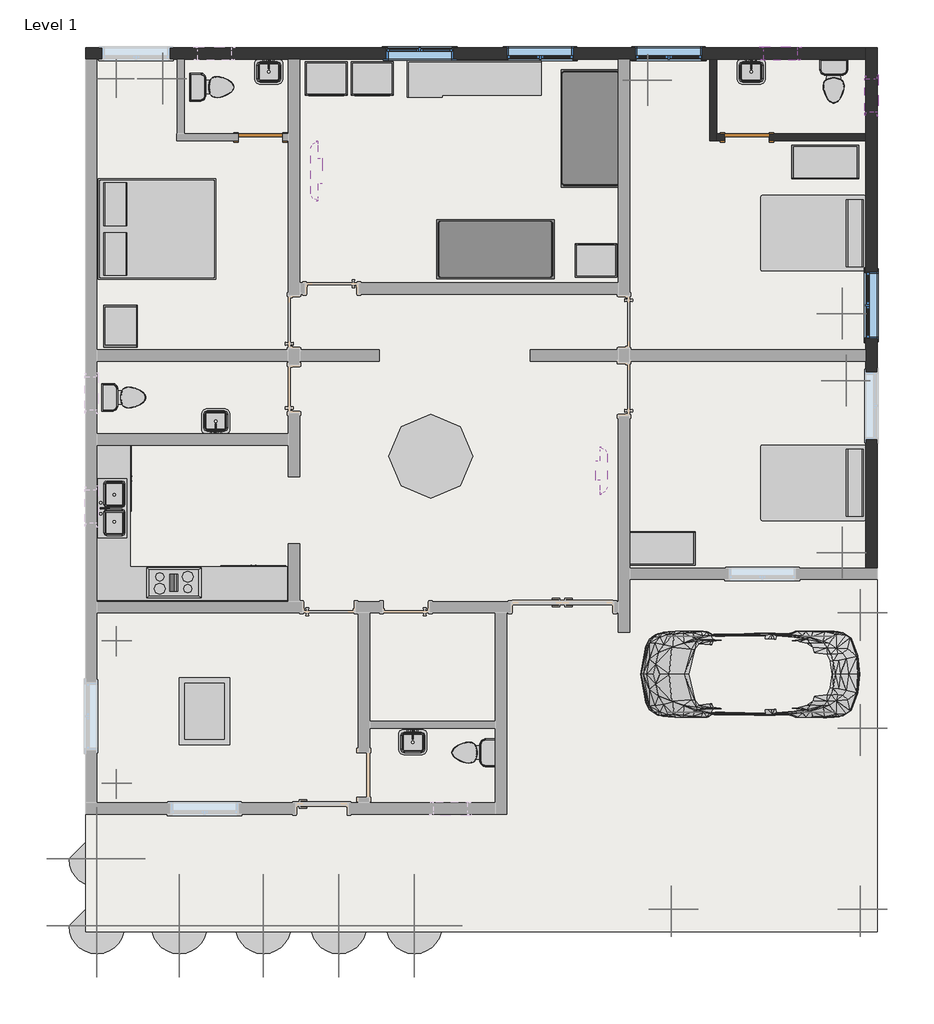
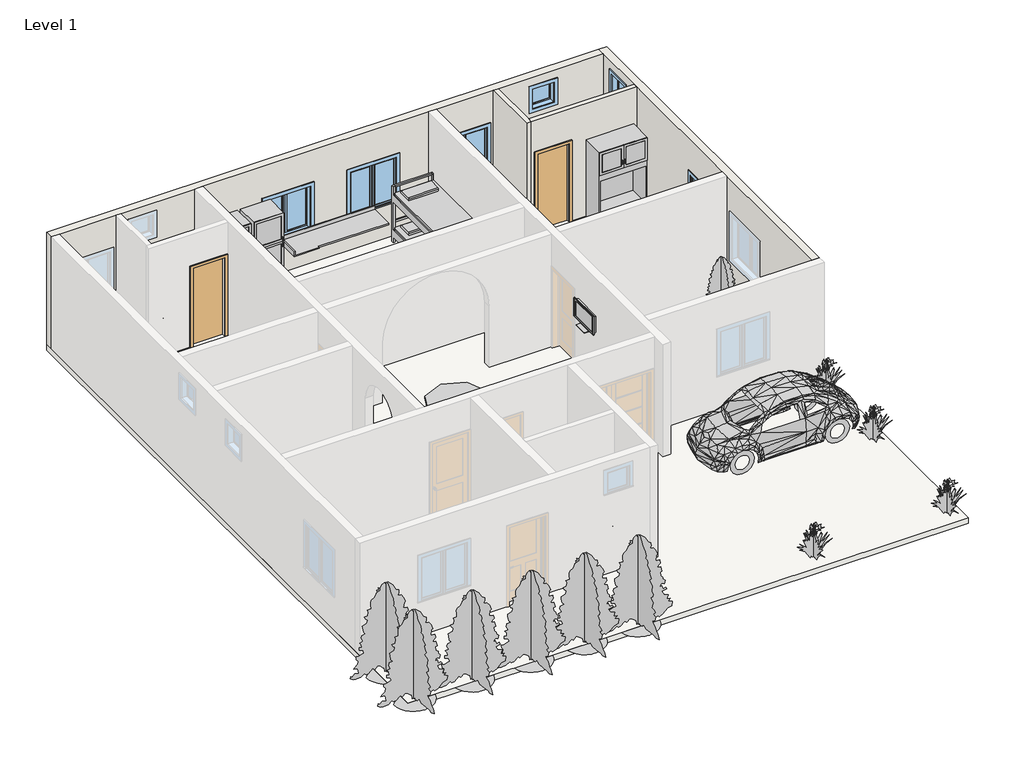
# One storey, part 2 of 2: 20 furniture elements, 18 geographic elements, 9 flow terminals, 6 windows, 4 walls, 2 doors, 2 proxies, 1 slab.
"""IFC4 building model written with IfcOpenShell, lengths in millimetres."""

from ifc_helpers import new_model, si_unit, frame, origin, place, context, project, spatial, polyline, outline, extrude, faceted_brep, transform, mapped, element, save
from components import cook_top_4_unit_30_51a8ed57, rpc_beetle_rpc_beetle_3ce7ba48, door_01e03998, door_af63d1be, flow_terminal_a53be723, flow_terminal_62a433f7, toilet_domestic_3d_toilet_domestic_3d_f7549cf7, toilet_domestic_3d_toilet_domestic_3d_183bbd19, furniture_7e5e5cd5, furniture_5816963c, furniture_2b620373, furniture_0253826f, furniture_3ce93e2e, furniture_bc267eac, furniture_56245f3a, furniture_7a3aaa4f, furniture_4da399da, furniture_bbcc68ce, tall_cabinet_2_door_built_in_3_fb6977ac, furniture_4aee2c20, furniture_7f1a6afb, rpc_plant_tropical_55f6ff97, rpc_tree_conifer_9dfc94cb, rpc_tree_conifer_8_e62f4ae5, rpc_tree_conifer_chinese_juniper_7_393522d0, rpc_tree_conifer_eastern_hemlock_25_66632feb, window_0862ab64, window_e41d21a6

model = new_model("IFC4")

# Units and contexts
model_context = context("Model", 3, world=origin())
ifc_project = project(units=[si_unit("LENGTHUNIT", "METRE", prefix="MILLI")], contexts=[model_context])

# Site, building, storey
site = spatial("IfcSite", under=ifc_project)
building = spatial("IfcBuilding", under=site)
storey = spatial("IfcBuildingStorey", under=building, Name="Level 1", Elevation=0.0)

# Proxies
placement = place(None, origin())
cook_top_4_unit_30_shape = cook_top_4_unit_30_51a8ed57(model_context)
element("IfcBuildingElementProxy", 1, Name="Cook Top-4 Unit : 30'", ObjectType="Cook Top-4 Unit : 30'", at=placement, inside=storey, context=model_context, shape_type="MappedRepresentation", body=[
    mapped(cook_top_4_unit_30_shape, transform((-1417.9231918, 1904.1987331, 152.4), x_axis=(1.0, 0.0, 0.0), y_axis=(0.0, 1.0, 0.0), z_axis=(0.0, 0.0, 1.0))),
])
rpc_beetle_rpc_beetle_shape = rpc_beetle_rpc_beetle_3ce7ba48(model_context)
element("IfcBuildingElementProxy", 2, Name="RPC Beetle : RPC Beetle", ObjectType="RPC Beetle : RPC Beetle", at=placement, inside=storey, context=model_context, shape_type="MappedRepresentation", body=[
    mapped(rpc_beetle_rpc_beetle_shape, transform((10291.4768082, 240.4987331, 0.0), x_axis=(0.0, 1.0, 0.0), y_axis=(-1.0, 0.0, 0.0), z_axis=(0.0, 0.0, 1.0))),
])

# Doors
door_shape = door_01e03998(model_context)
element("IfcDoor", 3, ObjectType="Door-Single-Panel : 32\" x 84\"", at=placement, inside=storey, context=model_context, shape_type="MappedRepresentation", body=[
    mapped(door_shape, transform((156.8768082, 9994.0987331, 0.0), x_axis=(1.0, 0.0, 0.0), y_axis=(0.0, 1.0, 0.0), z_axis=(0.0, 0.0, 1.0))),
])
door_2_shape = door_af63d1be(model_context)
element("IfcDoor", 4, ObjectType="Door-Single-Panel : 32\" x 84\"", at=placement, inside=storey, context=model_context, shape_type="MappedRepresentation", body=[
    mapped(door_2_shape, transform((8996.0768082, 9994.0987331, 0.0), x_axis=(-1.0, 0.0, 0.0), y_axis=(0.0, -1.0, 0.0), z_axis=(0.0, 0.0, 1.0))),
])

# Flow terminals
flow_terminal_shape = flow_terminal_a53be723(model_context)
element("IfcFlowTerminal", 5, ObjectType="Sink Kitchen-Double : 42\" x 21\"", at=placement, inside=storey, context=model_context, shape_type="MappedRepresentation", body=[
    mapped(flow_terminal_shape, transform((-2533.1777907, 3240.0622298, 0.0), x_axis=(0.0, 1.0, 0.0), y_axis=(-1.0, 0.0, 0.0), z_axis=(0.0, 0.0, 1.0))),
])
flow_terminal_2_shape = flow_terminal_62a433f7(model_context)
element("IfcFlowTerminal", 6, ObjectType="Sink Vanity-Square : 20\" x 18\"", at=placement, inside=storey, context=model_context, shape_type="MappedRepresentation", body=[
    mapped(flow_terminal_2_shape, transform((-640.2339512, 4789.4441342, 0.0), x_axis=(-1.0000000000000002, 0.0, 0.0), y_axis=(0.0, -1.0000000000000002, 0.0), z_axis=(0.0, 0.0, 1.0))),
])
element("IfcFlowTerminal", 7, ObjectType="Sink Vanity-Square : 20\" x 18\"", at=placement, inside=storey, context=model_context, shape_type="MappedRepresentation", body=[
    mapped(flow_terminal_2_shape, transform((293.5875676, 11236.353332, 0.0), x_axis=(1.0, 0.0, 0.0), y_axis=(0.0, 1.0, 0.0), z_axis=(0.0, 0.0, 1.0))),
])
element("IfcFlowTerminal", 8, ObjectType="Sink Vanity-Square : 20\" x 18\"", at=placement, inside=storey, context=model_context, shape_type="MappedRepresentation", body=[
    mapped(flow_terminal_2_shape, transform((9056.5875676, 11236.353332, 0.0), x_axis=(1.0, 0.0, 0.0), y_axis=(0.0, 1.0, 0.0), z_axis=(0.0, 0.0, 1.0))),
])
element("IfcFlowTerminal", 9, ObjectType="Sink Vanity-Square : 20\" x 18\"", at=placement, inside=storey, context=model_context, shape_type="MappedRepresentation", body=[
    mapped(flow_terminal_2_shape, transform((2909.7875676, -942.946668, 0.0), x_axis=(1.0, 0.0, 0.0), y_axis=(0.0, 1.0, 0.0), z_axis=(0.0, 0.0, 1.0))),
])
toilet_domestic_3d_toilet_domestic_3d_shape = toilet_domestic_3d_toilet_domestic_3d_f7549cf7(model_context)
toilet_domestic_3d_toilet_domestic_3d_2_shape = toilet_domestic_3d_toilet_domestic_3d_183bbd19(model_context)
element("IfcFlowTerminal", 10, ObjectType="Toilet-Domestic-3D : Toilet-Domestic-3D", at=placement, inside=storey, context=model_context, shape_type="MappedRepresentation", body=[
    mapped(toilet_domestic_3d_toilet_domestic_3d_shape, transform((3941.4768082, -1181.9012669, 0.0), x_axis=(0.0, -1.0, 0.0), y_axis=(1.0, 0.0, 0.0), z_axis=(0.0, 0.0, 1.0))),
    mapped(toilet_domestic_3d_toilet_domestic_3d_2_shape, transform((3941.4768082, -1181.9012669, 0.0), x_axis=(0.0, -1.0, 0.0), y_axis=(1.0, 0.0, 0.0), z_axis=(0.0, 0.0, 1.0))),
])
element("IfcFlowTerminal", 11, ObjectType="Toilet-Domestic-3D : Toilet-Domestic-3D", at=placement, inside=storey, context=model_context, shape_type="MappedRepresentation", body=[
    mapped(toilet_domestic_3d_toilet_domestic_3d_shape, transform((-630.5231918, 10908.4987331, 0.0), x_axis=(0.0, 1.0000000000000004, 0.0), y_axis=(-1.0000000000000004, 0.0, 0.0), z_axis=(0.0, 0.0, 1.0))),
    mapped(toilet_domestic_3d_toilet_domestic_3d_2_shape, transform((-630.5231918, 10908.4987331, 0.0), x_axis=(0.0, 1.0000000000000004, 0.0), y_axis=(-1.0000000000000004, 0.0, 0.0), z_axis=(0.0, 0.0, 1.0))),
])
element("IfcFlowTerminal", 12, ObjectType="Toilet-Domestic-3D : Toilet-Domestic-3D", at=placement, inside=storey, context=model_context, shape_type="MappedRepresentation", body=[
    mapped(toilet_domestic_3d_toilet_domestic_3d_shape, transform((10570.8768082, 10921.8027057, 0.0), x_axis=(1.0000000000000004, 0.0, 0.0), y_axis=(0.0, 1.0000000000000004, 0.0), z_axis=(0.0, 0.0, 1.0))),
    mapped(toilet_domestic_3d_toilet_domestic_3d_2_shape, transform((10570.8768082, 10921.8027057, 0.0), x_axis=(1.0000000000000004, 0.0, 0.0), y_axis=(0.0, 1.0000000000000004, 0.0), z_axis=(0.0, 0.0, 1.0))),
])
element("IfcFlowTerminal", 13, ObjectType="Toilet-Domestic-3D : Toilet-Domestic-3D", at=placement, inside=storey, context=model_context, shape_type="MappedRepresentation", body=[
    mapped(toilet_domestic_3d_toilet_domestic_3d_shape, transform((-2230.7231918, 5269.6987331, 0.0), x_axis=(0.0, 1.0, 0.0), y_axis=(-1.0, 0.0, 0.0), z_axis=(0.0, 0.0, 1.0))),
    mapped(toilet_domestic_3d_toilet_domestic_3d_2_shape, transform((-2230.7231918, 5269.6987331, 0.0), x_axis=(0.0, 1.0, 0.0), y_axis=(-1.0, 0.0, 0.0), z_axis=(0.0, 0.0, 1.0))),
])

# Furniture
furniture_shape = furniture_7e5e5cd5(model_context)
element("IfcFurniture", 14, ObjectType="48\"", at=placement, inside=storey, context=model_context, shape_type="MappedRepresentation", body=[
    mapped(furniture_shape, transform((120.7217682, 1586.6987331, 0.0), x_axis=(-1.0, 0.0, 0.0), y_axis=(0.0, -1.0, 0.0), z_axis=(0.0, 0.0, 1.0))),
])
element("IfcFurniture", 15, ObjectType="48\"", at=placement, inside=storey, context=model_context, shape_type="MappedRepresentation", body=[
    mapped(furniture_shape, transform((-1225.4782318, 1561.2987331, 0.0), x_axis=(-1.0, 0.0, 0.0), y_axis=(0.0, -1.0, 0.0), z_axis=(0.0, 0.0, 1.0))),
])
element("IfcFurniture", 16, ObjectType="48\"", at=placement, inside=storey, context=model_context, shape_type="MappedRepresentation", body=[
    mapped(furniture_shape, transform((-2814.9231918, 3705.6537731, 0.0), x_axis=(0.0, 1.0000000000000002, 0.0), y_axis=(-1.0000000000000002, 0.0, 0.0), z_axis=(0.0, 0.0, 1.0))),
])
furniture_2_shape = furniture_5816963c(model_context)
element("IfcFurniture", 17, ObjectType="82\" x 36\"", at=placement, inside=storey, context=model_context, shape_type="MappedRepresentation", body=[
    mapped(furniture_2_shape, transform((4033.0833656, 7553.6167659, 0.0), x_axis=(0.0, 1.0000000000000002, 0.0), y_axis=(-1.0000000000000002, 0.0, 0.0), z_axis=(0.0, 0.0, 1.0))),
])
element("IfcFurniture", 18, ObjectType="82\" x 36\"", at=placement, inside=storey, context=model_context, shape_type="MappedRepresentation", body=[
    mapped(furniture_2_shape, transform((5742.794841, 10550.1921757, 0.0), x_axis=(1.0, 0.0, 0.0), y_axis=(0.0, 1.0, 0.0), z_axis=(0.0, 0.0, 1.0))),
])
furniture_3_shape = furniture_2b620373(model_context)
element("IfcFurniture", 19, ObjectType="Bed-Box : Double 53\" x 74\"", at=placement, inside=storey, context=model_context, shape_type="MappedRepresentation", body=[
    mapped(furniture_3_shape, transform((-1957.1527, 7991.2462741, 0.0), x_axis=(0.0, 1.0000000000000002, 0.0), y_axis=(-1.0000000000000002, 0.0, 0.0), z_axis=(0.0, 0.0, 1.0))),
])
furniture_4_shape = furniture_0253826f(model_context)
element("IfcFurniture", 20, ObjectType="Bed-Standard : Double 54\" x 75\"", at=placement, inside=storey, context=model_context, shape_type="MappedRepresentation", body=[
    mapped(furniture_4_shape, transform((10248.1718902, 8525.6872577, 0.0), x_axis=(0.0, -1.0000000000000002, 0.0), y_axis=(1.0000000000000002, 0.0, 0.0), z_axis=(0.0, 0.0, 1.0))),
])
element("IfcFurniture", 21, ObjectType="Bed-Standard : Double 54\" x 75\"", at=placement, inside=storey, context=model_context, shape_type="MappedRepresentation", body=[
    mapped(furniture_4_shape, transform((10248.1718902, 3991.7872577, 0.0), x_axis=(0.0, -1.0, 0.0), y_axis=(1.0, 0.0, 0.0), z_axis=(0.0, 0.0, 1.0))),
])
furniture_5_shape = furniture_3ce93e2e(model_context)
element("IfcFurniture", 22, ObjectType="Counter Top-L Shaped : 24\" Depth", at=placement, inside=storey, context=model_context, shape_type="MappedRepresentation", body=[
    mapped(furniture_5_shape, transform((4024.3391033, 11391.0987331, 0.0), x_axis=(1.0, 0.0, 0.0), y_axis=(0.0, 1.0, 0.0), z_axis=(0.0, 0.0, 1.0))),
])
furniture_6_shape = furniture_bc267eac(model_context)
element("IfcFurniture", 23, ObjectType="Counter Top-L Shaped w Sink : 24\" Depth", at=placement, inside=storey, context=model_context, shape_type="MappedRepresentation", body=[
    mapped(furniture_6_shape, transform((-2840.3231918, 2761.7610282, 0.0), x_axis=(0.0, 1.0, 0.0), y_axis=(-1.0, 0.0, 0.0), z_axis=(0.0, 0.0, 1.0))),
])
furniture_7_shape = furniture_56245f3a(model_context)
element("IfcFurniture", 24, ObjectType="TV - Flat Screen : 32\"", at=placement, inside=storey, context=model_context, shape_type="MappedRepresentation", body=[
    mapped(furniture_7_shape, transform((6397.5381845, 3936.0550082, 1828.8), x_axis=(0.0, -1.0000000000000007, 0.0), y_axis=(1.0000000000000007, 0.0, 0.0), z_axis=(0.0, 0.0, 1.0))),
])
furniture_8_shape = furniture_7a3aaa4f(model_context)
element("IfcFurniture", 25, ObjectType="TV - Flat Screen : 42\"", at=placement, inside=storey, context=model_context, shape_type="MappedRepresentation", body=[
    mapped(furniture_8_shape, transform((1129.8154318, 9388.4432472, 1524.0), x_axis=(0.0, 1.0000000000000007, 0.0), y_axis=(-1.0000000000000007, 0.0, 0.0), z_axis=(0.0, 0.0, 1.0))),
])
furniture_9_shape = furniture_4da399da(model_context)
element("IfcFurniture", 26, ObjectType="Table-Coffee : 24\" x 24\" x 24\"", at=placement, inside=storey, context=model_context, shape_type="MappedRepresentation", body=[
    mapped(furniture_9_shape, transform((-763.912114, -450.8670336, 0.0), x_axis=(0.0, 1.0000000000000002, 0.0), y_axis=(-1.0000000000000002, 0.0, 0.0), z_axis=(0.0, 0.0, 1.0))),
])
furniture_10_shape = furniture_bbcc68ce(model_context)
element("IfcFurniture", 27, ObjectType="Table-Dining Round w Chairs : 36\" Diameter", at=placement, inside=storey, context=model_context, shape_type="MappedRepresentation", body=[
    mapped(furniture_10_shape, transform((3146.914841, 4387.7774216, 0.0), x_axis=(1.0, 0.0, 0.0), y_axis=(0.0, 1.0, 0.0), z_axis=(0.0, 0.0, 1.0))),
])
tall_cabinet_2_door_built_in_3_shape = tall_cabinet_2_door_built_in_3_fb6977ac(model_context)
element("IfcFurniture", 28, ObjectType="Tall Cabinet-2 Door-Built in : 3'", at=placement, inside=storey, context=model_context, shape_type="MappedRepresentation", body=[
    mapped(tall_cabinet_2_door_built_in_3_shape, transform((-2687.9231918, 6546.3610282, 0.0), x_axis=(0.0, 1.0, 0.0), y_axis=(-1.0, 0.0, 0.0), z_axis=(0.0, 0.0, 1.0))),
])
furniture_11_shape = furniture_4aee2c20(model_context)
element("IfcFurniture", 29, ObjectType="Tall Cabinet-2 Door-Built in : 30\"", at=placement, inside=storey, context=model_context, shape_type="MappedRepresentation", body=[
    mapped(furniture_11_shape, transform((7465.4145131, 2221.6987331, 0.0), x_axis=(-1.0, 0.0, 0.0), y_axis=(0.0, -1.0, 0.0), z_axis=(0.0, 0.0, 1.0))),
])
element("IfcFurniture", 30, ObjectType="Tall Cabinet-2 Door-Built in : 30\"", at=placement, inside=storey, context=model_context, shape_type="MappedRepresentation", body=[
    mapped(furniture_11_shape, transform((10399.7391033, 9854.3987331, 0.0), x_axis=(1.0000000000000002, 0.0, 0.0), y_axis=(0.0, 1.0000000000000002, 0.0), z_axis=(0.0, 0.0, 1.0))),
])
furniture_12_shape = furniture_7f1a6afb(model_context)
element("IfcFurniture", 31, ObjectType="Tall Cabinet-Single Door(2) : 30\"", at=placement, inside=storey, context=model_context, shape_type="MappedRepresentation", body=[
    mapped(furniture_12_shape, transform((1331.9391033, 11365.6987331, 0.0), x_axis=(1.0, 0.0, 0.0), y_axis=(0.0, 1.0, 0.0), z_axis=(0.0, 0.0, 1.0))),
])
element("IfcFurniture", 32, ObjectType="Tall Cabinet-Single Door(2) : 30\"", at=placement, inside=storey, context=model_context, shape_type="MappedRepresentation", body=[
    mapped(furniture_12_shape, transform((2170.1391033, 11365.6987331, 0.0), x_axis=(1.0, 0.0, 0.0), y_axis=(0.0, 1.0, 0.0), z_axis=(0.0, 0.0, 1.0))),
])
element("IfcFurniture", 33, ObjectType="Tall Cabinet-Single Door(2) : 30\"", at=placement, inside=storey, context=model_context, shape_type="MappedRepresentation", body=[
    mapped(furniture_12_shape, transform((6271.6145131, 7454.0987331, 0.0), x_axis=(-1.0, 0.0, 0.0), y_axis=(0.0, -1.0, 0.0), z_axis=(0.0, 0.0, 1.0))),
])

# Geographic elements
rpc_plant_tropical_shape = rpc_plant_tropical_55f6ff97(model_context)
element("IfcGeographicElement", 34, ObjectType="RPC Plant - Tropical", at=placement, inside=storey, context=model_context, shape_type="MappedRepresentation", body=[
    mapped(rpc_plant_tropical_shape, transform((7624.4768082, -4026.7012669, 0.0), x_axis=(1.0, 0.0, 0.0), y_axis=(0.0, 1.0, 0.0), z_axis=(0.0, 0.0, 1.0))),
])
element("IfcGeographicElement", 35, ObjectType="RPC Plant - Tropical", at=placement, inside=storey, context=model_context, shape_type="MappedRepresentation", body=[
    mapped(rpc_plant_tropical_shape, transform((11053.4768082, -4026.7012669, 0.0), x_axis=(1.0, 0.0, 0.0), y_axis=(0.0, 1.0, 0.0), z_axis=(0.0, 0.0, 1.0))),
])
element("IfcGeographicElement", 36, ObjectType="RPC Plant - Tropical", at=placement, inside=storey, context=model_context, shape_type="MappedRepresentation", body=[
    mapped(rpc_plant_tropical_shape, transform((11053.4768082, 1358.0987331, 0.0), x_axis=(1.0, 0.0, 0.0), y_axis=(0.0, 1.0, 0.0), z_axis=(0.0, 0.0, 1.0))),
])
element("IfcGeographicElement", 37, ObjectType="RPC Plant - Tropical", at=placement, inside=storey, context=model_context, shape_type="MappedRepresentation", body=[
    mapped(rpc_plant_tropical_shape, transform((11053.4768082, -737.4012669, 0.0), x_axis=(1.0, 0.0, 0.0), y_axis=(0.0, 1.0, 0.0), z_axis=(0.0, 0.0, 1.0))),
])
rpc_tree_conifer_shape = rpc_tree_conifer_9dfc94cb(model_context)
element("IfcGeographicElement", 38, ObjectType="RPC Tree - Conifer", at=placement, inside=storey, context=model_context, shape_type="MappedRepresentation", body=[
    mapped(rpc_tree_conifer_shape, transform((-2815.1198629, -4331.5012669, 0.0), x_axis=(1.0, 0.0, 0.0), y_axis=(0.0, 1.0, 0.0), z_axis=(0.0, 0.0, 1.0))),
])
element("IfcGeographicElement", 39, ObjectType="RPC Tree - Conifer", at=placement, inside=storey, context=model_context, shape_type="MappedRepresentation", body=[
    mapped(rpc_tree_conifer_shape, transform((-1316.5198629, -4331.5012669, 0.0), x_axis=(1.0, 0.0, 0.0), y_axis=(0.0, 1.0, 0.0), z_axis=(0.0, 0.0, 1.0))),
])
element("IfcGeographicElement", 40, ObjectType="RPC Tree - Conifer", at=placement, inside=storey, context=model_context, shape_type="MappedRepresentation", body=[
    mapped(rpc_tree_conifer_shape, transform((207.4801371, -4331.5012669, 0.0), x_axis=(1.0, 0.0, 0.0), y_axis=(0.0, 1.0, 0.0), z_axis=(0.0, 0.0, 1.0))),
])
element("IfcGeographicElement", 41, ObjectType="RPC Tree - Conifer", at=placement, inside=storey, context=model_context, shape_type="MappedRepresentation", body=[
    mapped(rpc_tree_conifer_shape, transform((1579.0801371, -4331.5012669, 0.0), x_axis=(1.0, 0.0, 0.0), y_axis=(0.0, 1.0, 0.0), z_axis=(0.0, 0.0, 1.0))),
])
element("IfcGeographicElement", 42, ObjectType="RPC Tree - Conifer", at=placement, inside=storey, context=model_context, shape_type="MappedRepresentation", body=[
    mapped(rpc_tree_conifer_shape, transform((2950.6801371, -4331.5012669, 0.0), x_axis=(1.0, 0.0, 0.0), y_axis=(0.0, 1.0, 0.0), z_axis=(0.0, 0.0, 1.0))),
])
element("IfcGeographicElement", 43, ObjectType="RPC Tree - Conifer", at=placement, inside=storey, context=model_context, shape_type="MappedRepresentation", body=[
    mapped(rpc_tree_conifer_shape, transform((-2815.1198629, -3112.3012669, 0.0), x_axis=(1.0, 0.0, 0.0), y_axis=(0.0, 1.0, 0.0), z_axis=(0.0, 0.0, 1.0))),
])
rpc_tree_conifer_8_shape = rpc_tree_conifer_8_e62f4ae5(model_context)
element("IfcGeographicElement", 44, ObjectType="RPC Tree - Conifer : 8'", at=placement, inside=storey, context=model_context, shape_type="MappedRepresentation", body=[
    mapped(rpc_tree_conifer_8_shape, transform((-1621.3198629, 11060.8987331, 0.0), x_axis=(1.0, 0.0, 0.0), y_axis=(0.0, 1.0, 0.0), z_axis=(0.0, 0.0, 1.0))),
])
rpc_tree_conifer_chinese_juniper_7_shape = rpc_tree_conifer_chinese_juniper_7_393522d0(model_context)
element("IfcGeographicElement", 45, ObjectType="RPC Tree - Conifer : Chinese Juniper - 7'", at=placement, inside=storey, context=model_context, shape_type="MappedRepresentation", body=[
    mapped(rpc_tree_conifer_chinese_juniper_7_shape, transform((-2459.5198629, -1740.7012669, 0.0), x_axis=(1.0, 0.0, 0.0), y_axis=(0.0, 1.0, 0.0), z_axis=(0.0, 0.0, 1.0))),
])
element("IfcGeographicElement", 46, ObjectType="RPC Tree - Conifer : Chinese Juniper - 7'", at=placement, inside=storey, context=model_context, shape_type="MappedRepresentation", body=[
    mapped(rpc_tree_conifer_chinese_juniper_7_shape, transform((-2459.5198629, 850.0987331, 0.0), x_axis=(1.0, 0.0, 0.0), y_axis=(0.0, 1.0, 0.0), z_axis=(0.0, 0.0, 1.0))),
])
rpc_tree_conifer_eastern_hemlock_25_shape = rpc_tree_conifer_eastern_hemlock_25_66632feb(model_context)
element("IfcGeographicElement", 47, ObjectType="RPC Tree - Conifer : Eastern Hemlock - 25'", at=placement, inside=storey, context=model_context, shape_type="MappedRepresentation", body=[
    mapped(rpc_tree_conifer_eastern_hemlock_25_shape, transform((-2459.5198629, 11060.8987331, 0.0), x_axis=(1.0, 0.0, 0.0), y_axis=(0.0, 1.0, 0.0), z_axis=(0.0, 0.0, 1.0))),
])
element("IfcGeographicElement", 48, ObjectType="RPC Tree - Conifer : r", at=placement, inside=storey, context=model_context, shape_type="MappedRepresentation", body=[
    mapped(rpc_tree_conifer_8_shape, transform((10723.0801371, 2450.2987331, 0.0), x_axis=(1.0, 0.0, 0.0), y_axis=(0.0, 1.0, 0.0), z_axis=(0.0, 0.0, 1.0))),
])
element("IfcGeographicElement", 49, ObjectType="RPC Tree - Conifer : t", at=placement, inside=storey, context=model_context, shape_type="MappedRepresentation", body=[
    mapped(rpc_tree_conifer_8_shape, transform((10723.0801371, 6793.6987331, 0.0), x_axis=(1.0, 0.0, 0.0), y_axis=(0.0, 1.0, 0.0), z_axis=(0.0, 0.0, 1.0))),
])
element("IfcGeographicElement", 50, ObjectType="RPC Tree - Conifer : t", at=placement, inside=storey, context=model_context, shape_type="MappedRepresentation", body=[
    mapped(rpc_tree_conifer_8_shape, transform((7192.4801371, 11035.4987331, 0.0), x_axis=(1.0, 0.0, 0.0), y_axis=(0.0, 1.0, 0.0), z_axis=(0.0, 0.0, 1.0))),
])
element("IfcGeographicElement", 51, ObjectType="RPC Tree - Conifer : y", at=placement, inside=storey, context=model_context, shape_type="MappedRepresentation", body=[
    mapped(rpc_tree_conifer_8_shape, transform((10799.2801371, 5574.4987331, 0.0), x_axis=(1.0, 0.0, 0.0), y_axis=(0.0, 1.0, 0.0), z_axis=(0.0, 0.0, 1.0))),
])

# Slab
element("IfcSlab", 52, ObjectType="Generic - 12\"", at=placement, inside=storey, context=model_context, shape_type="SweptSolid", body=[
    extrude(outline(polyline([(11358.2768082, 11619.6987331), (11358.2768082, -4433.1012669), (-3018.1231918, -4433.1012669), (-3018.1231918, 11619.6987331), (11358.2768082, 11619.6987331)])), frame((0.0, 0.0, -152.4), z_axis=(0.0, 0.0, 1.0), x_axis=(1.0, 0.0, 0.0)), (0.0, 0.0, 1.0), 152.4),
])

# Walls
element("IfcWall", 53, ObjectType="Generic - 5\"", at=placement, inside=storey, context=model_context, shape_type="SweptSolid", body=[
    extrude(outline(polyline([(0.0, 8449.9768082), (0.0, 8589.6768082), (2133.6, 8589.6768082), (2133.6, 9402.4768082), (0.0, 9402.4768082), (0.0, 11155.0768082), (3048.0, 11155.0768082), (3048.0, 8449.9768082), (0.0, 8449.9768082)])), frame((0.0, 9930.5987331, 0.0), z_axis=(0.0, 1.0, 0.0), x_axis=(0.0, 0.0, 1.0)), (0.0, 0.0, 1.0), 127.0),
])
element("IfcWall", 54, ObjectType="Generic - 5\"", at=placement, inside=storey, context=model_context, shape_type="Brep", body=[
    faceted_brep([(8322.9768082, 11416.4987331, 0.0), (8322.9768082, 9930.5987331, 0.0), (8322.9768082, 9930.5987331, 3048.0), (8322.9768082, 11416.4987331, 3048.0), (8449.9768082, 11416.4987331, 0.0), (8449.9768082, 11416.4987331, 3048.0), (8449.9768082, 10057.5987331, 3048.0), (8449.9768082, 9930.5987331, 3048.0), (8449.9768082, 9930.5987331, 0.0), (8449.9768082, 10057.5987331, 0.0)], [[[0, 1, 2, 3]], [[4, 5, 6, 7, 8, 9]], [[1, 0, 4, 9, 8]], [[3, 2, 7, 6, 5]], [[0, 3, 5, 4]], [[2, 1, 8, 7]]]),
])
element("IfcWall", 55, ObjectType="Generic - 8\"", at=placement, inside=storey, context=model_context, shape_type="Brep", body=[
    faceted_brep([(-3018.1231918, 11416.4987331, 0.0), (-2814.9231918, 11416.4987331, 0.0), (-1354.4231918, 11416.4987331, 0.0), (-1227.4231918, 11416.4987331, 0.0), (664.8768082, 11416.4987331, 0.0), (868.0768082, 11416.4987331, 0.0), (6659.2768082, 11416.4987331, 0.0), (6862.4768082, 11416.4987331, 0.0), (8322.9768082, 11416.4987331, 0.0), (8449.9768082, 11416.4987331, 0.0), (11155.0768082, 11416.4987331, 0.0), (11155.0768082, 11416.4987331, 3048.0), (8449.9768082, 11416.4987331, 3048.0), (8322.9768082, 11416.4987331, 3048.0), (6862.4768082, 11416.4987331, 3048.0), (6659.2768082, 11416.4987331, 3048.0), (868.0768082, 11416.4987331, 3048.0), (664.8768082, 11416.4987331, 3048.0), (-1227.4231918, 11416.4987331, 3048.0), (-1354.4231918, 11416.4987331, 3048.0), (-2814.9231918, 11416.4987331, 3048.0), (-3018.1231918, 11416.4987331, 3048.0), (-2713.3231918, 11416.4987331, 2133.6), (-1494.1231918, 11416.4987331, 2133.6), (-1494.1231918, 11416.4987331, 914.4), (-2713.3231918, 11416.4987331, 914.4), (3662.0768082, 11416.4987331, 2133.6), (3662.0768082, 11416.4987331, 914.4), (2442.8768082, 11416.4987331, 914.4), (2442.8768082, 11416.4987331, 2133.6), (4627.2768082, 11416.4987331, 2133.6), (5846.4768082, 11416.4987331, 2133.6), (5846.4768082, 11416.4987331, 914.4), (4627.2768082, 11416.4987331, 914.4), (6964.0768082, 11416.4987331, 2133.6), (8183.2768082, 11416.4987331, 2133.6), (8183.2768082, 11416.4987331, 914.4), (6964.0768082, 11416.4987331, 914.4), (9910.4768082, 11416.4987331, 2768.6), (9910.4768082, 11416.4987331, 2159.0), (9300.8768082, 11416.4987331, 2159.0), (9300.8768082, 11416.4987331, 2768.6), (-376.5231918, 11416.4987331, 2768.6), (-376.5231918, 11416.4987331, 2159.0), (-986.1231918, 11416.4987331, 2159.0), (-986.1231918, 11416.4987331, 2768.6), (-3018.1231918, 11619.6987331, 0.0), (-3018.1231918, 11619.6987331, 3048.0), (11155.0768082, 11619.6987331, 3048.0), (11155.0768082, 11619.6987331, 0.0), (-2713.3231918, 11619.6987331, 2133.6), (-2713.3231918, 11619.6987331, 914.4), (-1494.1231918, 11619.6987331, 914.4), (-1494.1231918, 11619.6987331, 2133.6), (3662.0768082, 11619.6987331, 2133.6), (2442.8768082, 11619.6987331, 2133.6), (2442.8768082, 11619.6987331, 914.4), (3662.0768082, 11619.6987331, 914.4), (4627.2768082, 11619.6987331, 2133.6), (4627.2768082, 11619.6987331, 914.4), (5846.4768082, 11619.6987331, 914.4), (5846.4768082, 11619.6987331, 2133.6), (6964.0768082, 11619.6987331, 2133.6), (6964.0768082, 11619.6987331, 914.4), (8183.2768082, 11619.6987331, 914.4), (8183.2768082, 11619.6987331, 2133.6), (9910.4768082, 11619.6987331, 2768.6), (9300.8768082, 11619.6987331, 2768.6), (9300.8768082, 11619.6987331, 2159.0), (9910.4768082, 11619.6987331, 2159.0), (-376.5231918, 11619.6987331, 2768.6), (-986.1231918, 11619.6987331, 2768.6), (-986.1231918, 11619.6987331, 2159.0), (-376.5231918, 11619.6987331, 2159.0)], [[[0, 1, 2, 3, 4, 5, 6, 7, 8, 9, 10, 11, 12, 13, 14, 15, 16, 17, 18, 19, 20, 21], [22, 23, 24, 25], [26, 27, 28, 29], [30, 31, 32, 33], [34, 35, 36, 37], [38, 39, 40, 41], [42, 43, 44, 45]], [[46, 47, 48, 49], [50, 51, 52, 53], [54, 55, 56, 57], [58, 59, 60, 61], [62, 63, 64, 65], [66, 67, 68, 69], [70, 71, 72, 73]], [[10, 9, 8, 7, 6, 5, 4, 3, 2, 1, 0, 46, 49]], [[21, 20, 19, 18, 17, 16, 15, 14, 13, 12, 11, 48, 47]], [[0, 21, 47, 46]], [[11, 10, 49, 48]], [[51, 50, 22, 25]], [[52, 51, 25, 24]], [[53, 52, 24, 23]], [[50, 53, 23, 22]], [[27, 26, 54, 57]], [[28, 27, 57, 56]], [[29, 28, 56, 55]], [[26, 29, 55, 54]], [[59, 58, 30, 33]], [[60, 59, 33, 32]], [[61, 60, 32, 31]], [[58, 61, 31, 30]], [[63, 62, 34, 37]], [[64, 63, 37, 36]], [[65, 64, 36, 35]], [[62, 65, 35, 34]], [[39, 38, 66, 69]], [[40, 39, 69, 68]], [[41, 40, 68, 67]], [[38, 41, 67, 66]], [[43, 42, 70, 73]], [[44, 43, 73, 72]], [[45, 44, 72, 71]], [[42, 45, 71, 70]]]),
])
element("IfcWall", 56, ObjectType="Generic - 8\"", at=placement, inside=storey, context=model_context, shape_type="Brep", body=[
    faceted_brep([(11155.0768082, 11619.6987331, 0.0), (11155.0768082, 11416.4987331, 0.0), (11155.0768082, 10057.5987331, 0.0), (11155.0768082, 9930.5987331, 0.0), (11155.0768082, 6133.2987331, 0.0), (11155.0768082, 5930.0987331, 0.0), (11155.0768082, 2170.8987331, 0.0), (11155.0768082, 2170.8987331, 3048.0), (11155.0768082, 5930.0987331, 3048.0), (11155.0768082, 6133.2987331, 3048.0), (11155.0768082, 9930.5987331, 3048.0), (11155.0768082, 10057.5987331, 3048.0), (11155.0768082, 11416.4987331, 3048.0), (11155.0768082, 11619.6987331, 3048.0), (11155.0768082, 7555.6987331, 2133.6), (11155.0768082, 6336.4987331, 2133.6), (11155.0768082, 6336.4987331, 914.4), (11155.0768082, 7555.6987331, 914.4), (11155.0768082, 4507.6987331, 2133.6), (11155.0768082, 4507.6987331, 914.4), (11155.0768082, 5726.8987331, 914.4), (11155.0768082, 5726.8987331, 2133.6), (11155.0768082, 10451.2987331, 2768.6), (11155.0768082, 10451.2987331, 2159.0), (11155.0768082, 11060.8987331, 2159.0), (11155.0768082, 11060.8987331, 2768.6), (11358.2768082, 11619.6987331, 0.0), (11358.2768082, 11619.6987331, 3048.0), (11358.2768082, 2170.8987331, 3048.0), (11358.2768082, 2170.8987331, 0.0), (11358.2768082, 7555.6987331, 2133.6), (11358.2768082, 7555.6987331, 914.4), (11358.2768082, 6336.4987331, 914.4), (11358.2768082, 6336.4987331, 2133.6), (11358.2768082, 4507.6987331, 2133.6), (11358.2768082, 5726.8987331, 2133.6), (11358.2768082, 5726.8987331, 914.4), (11358.2768082, 4507.6987331, 914.4), (11358.2768082, 10451.2987331, 2768.6), (11358.2768082, 11060.8987331, 2768.6), (11358.2768082, 11060.8987331, 2159.0), (11358.2768082, 10451.2987331, 2159.0)], [[[0, 1, 2, 3, 4, 5, 6, 7, 8, 9, 10, 11, 12, 13], [14, 15, 16, 17], [18, 19, 20, 21], [22, 23, 24, 25]], [[26, 27, 28, 29], [30, 31, 32, 33], [34, 35, 36, 37], [38, 39, 40, 41]], [[6, 5, 4, 3, 2, 1, 0, 26, 29]], [[13, 12, 11, 10, 9, 8, 7, 28, 27]], [[0, 13, 27, 26]], [[7, 6, 29, 28]], [[31, 30, 14, 17]], [[32, 31, 17, 16]], [[33, 32, 16, 15]], [[30, 33, 15, 14]], [[19, 18, 34, 37]], [[20, 19, 37, 36]], [[21, 20, 36, 35]], [[18, 21, 35, 34]], [[23, 22, 38, 41]], [[24, 23, 41, 40]], [[25, 24, 40, 39]], [[22, 25, 39, 38]]]),
])

# Windows
window_shape = window_0862ab64(model_context)
element("IfcWindow", 57, ObjectType="Casement Dbl with Trim : 48\" x 48\"", at=placement, inside=storey, context=model_context, shape_type="MappedRepresentation", body=[
    mapped(window_shape, transform((3052.4768082, 11499.0487331, 0.0), x_axis=(1.0, 0.0, 0.0), y_axis=(0.0, 1.0, 0.0), z_axis=(0.0, 0.0, 1.0))),
])
element("IfcWindow", 58, ObjectType="Casement Dbl with Trim : 48\" x 48\"", at=placement, inside=storey, context=model_context, shape_type="MappedRepresentation", body=[
    mapped(window_shape, transform((5236.8768082, 11537.1487331, 0.0), x_axis=(-1.0, 0.0, 0.0), y_axis=(0.0, -1.0, 0.0), z_axis=(0.0, 0.0, 1.0))),
])
element("IfcWindow", 59, ObjectType="Casement Dbl with Trim : 48\" x 48\"", at=placement, inside=storey, context=model_context, shape_type="MappedRepresentation", body=[
    mapped(window_shape, transform((7573.6768082, 11537.1487331, 0.0), x_axis=(-1.0, 0.0, 0.0), y_axis=(0.0, -1.0, 0.0), z_axis=(0.0, 0.0, 1.0))),
])
element("IfcWindow", 60, ObjectType="Casement Dbl with Trim : 48\" x 48\"", at=placement, inside=storey, context=model_context, shape_type="MappedRepresentation", body=[
    mapped(window_shape, transform((11275.7268082, 6946.0987331, 0.0), x_axis=(0.0, 1.0, 0.0), y_axis=(-1.0, 0.0, 0.0), z_axis=(0.0, 0.0, 1.0))),
])
window_2_shape = window_e41d21a6(model_context)
element("IfcWindow", 61, ObjectType="Transom with Trim : 24\" x 24\"", at=placement, inside=storey, context=model_context, shape_type="MappedRepresentation", body=[
    mapped(window_2_shape, transform((9643.7768082, 11518.0987331, 0.0), x_axis=(1.0, 0.0, 0.0), y_axis=(0.0, 1.0, 0.0), z_axis=(0.0, 0.0, 1.0))),
])
element("IfcWindow", 62, ObjectType="Transom with Trim : 24\" x 24\"", at=placement, inside=storey, context=model_context, shape_type="MappedRepresentation", body=[
    mapped(window_2_shape, transform((11256.6768082, 10717.9987331, 0.0), x_axis=(0.0, -1.0, 0.0), y_axis=(1.0, 0.0, 0.0), z_axis=(0.0, 0.0, 1.0))),
])

save(model, "model.ifc")

# Revit data of these elements
# Type "Cook Top-4 Unit : 30'"
#   Assembly Code = "E1090400"
#   Depth = 1' - 6 123/256"
#   Width = 3' - 0"
#   Burner Material = Steel, Chrome Plated
#   Cooktop Material = Steel, Polished
#   Default Elevation = 0
# Type "RPC Beetle : RPC Beetle"
#   built-in parameter 1005195 = "RPC-16-0U6E-L4EG-ENH1-J3KF-SVEL-0TX4-C0"
#   Height = 0
# Type "Door-Single-Panel : 32\" x 84\""
#   Type Mark = "11"
#   Construction Type Id = "DOOR"
#   Assembly Code = "C1020300"
#   Analytic Construction = "Wooden"
#   Thickness = 0' - 2"
#   Thermal Resistance (R) = 2.5876 (h·ft²·°F)/BTU
#   Swing Angle [instance default] = 90.00°
#   Heat Transfer Coefficient (U) = 0.3865 BTU/(h·ft²·°F)
#   Height = 7' - 0"
#   Trim Projection Ext = 0' - 1"
#   Trim Projection Int = 0' - 1"
#   Trim Width = 0' - 3"
#   Width = 2' - 8"
#   Define Thermal Properties by = 1
#   Panel Material = Wood - Birch - Solid Stained Light Low Gloss
#   Trim Material = Paint - Sienna
#   Visual Light Transmittance = 0
#   Solar Heat Gain Coefficient = 0
#   Function = (empty or 0)
#   Wall Closure = (empty or 0)
# Type "Sink Kitchen-Double : 42\" x 21\""
#   Assembly Code = "D2010410"
#   Counter Height = 3' - 0"
#   Depth = 1' - 9"
#   Width = 3' - 6"
#   Faucet Material = Steel, Polished
#   Sink Material = Steel, Polished
#   Default Elevation = 0
# Type "Sink Vanity-Square : 20\" x 18\""
#   Assembly Code = "D2010400"
#   Counter Height = 2' - 7"
#   Depth = 1' - 6"
#   Width = 1' - 8"
#   Basin Material = Porcelain, Linen
#   Faucet Material = Steel, Polished
#   Default Elevation = 0
# Type "Toilet-Domestic-3D : Toilet-Domestic-3D"
#   Assembly Code = "D2010110"
#   Toilet - Bowl/Basin Material = Porcelain, Linen
#   Toilet - Seat Material = Laminate, Linen, Matte
#   Default Elevation = 0
# Type "48\""
#   Assembly Code = "C1030410"
#   Depth = 2' - 0"
#   Height = 2' - 5 1/2"
#   Toe Depth = 0' - 3"
#   Toe Height = 0' - 3 1/2"
#   Width = 4' - 0"
#   Cabinet Material = none
#   Door/Drawer Material = none
#   Handle Material = Cabinets - Handles
#   Default Elevation = 0
# Type "82\" x 36\""
#   Assembly Code = "E2020200"
#   Height = 5' - 0"
#   Length = 7' - 0"
#   Width = 3' - 6"
#   Frame Material = Birch
#   Mattress Material = Linen, White
#   Default Elevation = 0
# Type "Bed-Box : Double 53\" x 74\""
#   Assembly Code = "E2020200"
#   Length = 7' - 0"
#   Width = 6' - 0"
#   Frame Material = Birch
#   Mattress Material = Linen, White
#   Default Elevation = 0
# Type "Bed-Standard : Double 54\" x 75\""
#   Assembly Code = "E2020200"
#   Length = 6' - 3"
#   Width = 4' - 6"
#   Leg Material = Steel, Chrome Plated
#   Mattress Material = Linen, White
#   Default Elevation = 0
# Type "Counter Top-L Shaped : 24\" Depth"
#   Assembly Code = "C1030400"
#   Counter Thickness = 0' - 1 1/2"
#   Depth = 2' - 1"
#   Height = 3' - 0"
#   Length - Leg 1 [instance default] = 8' - 0"
#   Length - Leg 2 [instance default] = 6' - 0"
#   Counter Top Material = none
#   Default Elevation = 0
# Type "Counter Top-L Shaped w Sink : 24\" Depth"
#   Assembly Code = "C1030400"
#   Counter Thickness = 0' - 1 1/2"
#   Depth = 2' - 1"
#   Height = 3' - 0"
#   Length - Leg 1 [instance default] = 8' - 0"
#   Length - Leg 2 [instance default] = 6' - 0"
#   Sink Location [instance default] = 3' - 0"
#   Sink Location To Wall [instance default] = 0' - 6"
#   Sink Opening Depth [instance default] = 1' - 3"
#   Sink Opening Width [instance default] = 3' - 3"
#   Counter Top Material = none
#   Default Elevation = 0
# Type "TV - Flat Screen : 32\""
#   SinAng = 0' - 0.0193"
#   L = 2' - 3.79372"
#   H = 1' - 3.6354"
#   Thickness = 0' - 4.33071"
#   Diagonal = 2' - 7.88976"
#   CosAng = 0' - 0.03431"
#   Stand [instance default] = yes
#   Default Elevation = 0
# Type "TV - Flat Screen : 42\""
#   SinAng = 0' - 0.0193"
#   L = 3' - 0.71517"
#   H = 1' - 8.65418"
#   Thickness = 0' - 4.33071"
#   Diagonal = 3' - 6.12598"
#   CosAng = 0' - 0.03431"
#   Stand [instance default] = yes
#   Default Elevation = 0
# Type "Table-Coffee : 24\" x 24\" x 24\""
#   Assembly Code = "E2020200"
#   Height = 2' - 0"
#   Length = 4' - 0"
#   Width = 3' - 0"
#   Top Material = none
#   Frame Material = none
#   Default Elevation = 0
# Type "Table-Dining Round w Chairs : 36\" Diameter"
#   Assembly Code = "E2020200"
#   Radius = 2' - 6"
#   Diameter = 5' - 0"
#   Height = 2' - 6"
#   Chairs = 8
#   Base Material = Pine
#   Top Material = Laminate, Linen, Matte
#   Default Elevation = 0
# Type "Tall Cabinet-2 Door-Built in : 3'"
#   Assembly Code = "C1030410"
#   Height = 7' - 0"
#   Depth = 2' - 0"
#   Height-Base of Built-in = 1' - 2"
#   Height-Built-in = 3' - 3 1/4"
#   Height-Upper Cabinet = 2' - 0"
#   Toe Depth = 0' - 3"
#   Toe Height = 0' - 3 1/2"
#   Width = 2' - 6"
#   Cabinet Material = none
#   Door/Drawer Material = none
#   Handle Material = Cabinets - Handles
#   Panel Material = Glass
#   Default Elevation = 0
#   Type Comments = ""
# Type "Tall Cabinet-2 Door-Built in : 30\""
#   Assembly Code = "C1030410"
#   Height = 7' - 0"
#   Depth = 2' - 0"
#   Height-Base of Built-in = 1' - 2"
#   Height-Built-in = 3' - 3 1/4"
#   Height-Upper Cabinet = 2' - 0"
#   Toe Depth = 0' - 3"
#   Toe Height = 0' - 3 1/2"
#   Width = 4' - 0"
#   Cabinet Material = none
#   Door/Drawer Material = none
#   Handle Material = Cabinets - Handles
#   Panel Material = Glass
#   Default Elevation = 0
#   Type Comments = ""
# Type "Tall Cabinet-Single Door(2) : 30\""
#   Assembly Code = "C1030410"
#   Depth = 2' - 0"
#   Height = 7' - 0"
#   Toe Depth = 0' - 3"
#   Toe Height = 0' - 3 1/2"
#   Width = 2' - 6"
#   Cabinet Material = none
#   Door/Drawer Material = none
#   Handle Material = Cabinets - Handles
#   Panel Material = none
#   Default Elevation = 0
# Type "RPC Plant - Tropical"
#   built-in parameter 1005198 = "{2, 15},{39, RPC-16-FWM5-GM7X-C67P-4000-ST1L-LVER-AU},{1, 0},{1, 0},{2, 13},{1, 8},{5, Color},{1, 0},{1, 0},{3, 0.8},{3, 0.8},{3, 0.8},{1, 8},{7, BBoxMin},{1, 0},{1, 0},{1, 0},{1, 0},{1, 0},{1, 8},{7, BBoxMax},{1, 0},{1, 0},{1, 0},{1, 0},{1, 0},{2, 11},{9, RPCTypeId},{1, 0},{1, 0},{39, RPC-16-FWM5-GM7X-C67P-4000-ST1L-LVER-AU},{1, 6},{14, RPCPlantHeight},{1, 0},{1, 0},{1, 3},{2, 11},{7, keyword},{1, 0},{1, 0},{35, :RPCs:Shrubs [General]:Geometry:RPC},{2, 11},{8, category},{1, 0},{1, 0},{16, Shrubs [General]},{2, 11},{12, LocalizedUID},{1, 0},{1, 0},{10, Crane Lily},{2, 14},{6, Height},{1, 0},{1, 0},{1, 3},{1, 2},{16, Cast Reflections},{1, 0},{1, 0},{1, 0},{1, 2},{12, Cast Shadows},{1, 0},{1, 0},{1, 1},{1, 2},{9, Lock View},{1, 0},{1, 0},{1, 0},{1, 4},{5, ViewC},{1, 0},{1, 0},{1, 0},{21, assetlibrary_base.fbx},{1, 5},"
#   built-in parameter 1005195 = "RPC-16-FWM5-GM7X-C67P-4000-ST1L-LVER-AU"
#   Assembly Code = "G2050500"
#   Height = 3' - 0"
#   Default Elevation = 0
# Type "RPC Tree - Conifer"
#   built-in parameter 1005198 = "{2, 15},{39, RPC-16-G0M4-N9PX-U6TN-C000-ST1L-LVER-AU},{1, 0},{1, 0},{2, 13},{1, 8},{5, Color},{1, 0},{1, 0},{3, 0.8},{3, 0.8},{3, 0.8},{1, 8},{7, BBoxMin},{1, 0},{1, 0},{1, 0},{1, 0},{1, 0},{1, 8},{7, BBoxMax},{1, 0},{1, 0},{1, 0},{1, 0},{1, 0},{2, 11},{9, RPCTypeId},{1, 0},{1, 0},{39, RPC-16-G0M4-N9PX-U6TN-C000-ST1L-LVER-AU},{1, 6},{14, RPCPlantHeight},{1, 0},{1, 0},{2, 13},{2, 11},{7, keyword},{1, 0},{1, 0},{34, :RPCs:Trees [General]:Geometry:RPC},{2, 11},{8, category},{1, 0},{1, 0},{15, Trees [General]},{2, 11},{12, LocalizedUID},{1, 0},{1, 0},{15, Colorado Spruce},{2, 14},{6, Height},{1, 0},{1, 0},{2, 13},{1, 2},{16, Cast Reflections},{1, 0},{1, 0},{1, 0},{1, 2},{12, Cast Shadows},{1, 0},{1, 0},{1, 1},{1, 2},{9, Lock View},{1, 0},{1, 0},{1, 0},{1, 4},{5, ViewC},{1, 0},{1, 0},{1, 0},{21, assetlibrary_base.fbx},{1, 5},"
#   built-in parameter 1005195 = "RPC-16-G0M4-N9PX-U6TN-C000-ST1L-LVER-AU"
#   Assembly Code = "G2050500"
#   Height = 8' - 0"
#   Description = (empty or 0)
#   Default Elevation = 0
# Type "RPC Tree - Conifer : 8'"
#   built-in parameter 1005198 = "{2, 15},{39, RPC-16-G0M4-N9PX-U6TN-C000-ST1L-LVER-AU},{1, 0},{1, 0},{2, 13},{1, 8},{5, Color},{1, 0},{1, 0},{3, 0.8},{3, 0.8},{3, 0.8},{1, 8},{7, BBoxMin},{1, 0},{1, 0},{1, 0},{1, 0},{1, 0},{1, 8},{7, BBoxMax},{1, 0},{1, 0},{1, 0},{1, 0},{1, 0},{2, 11},{9, RPCTypeId},{1, 0},{1, 0},{39, RPC-16-G0M4-N9PX-U6TN-C000-ST1L-LVER-AU},{1, 6},{14, RPCPlantHeight},{1, 0},{1, 0},{2, 13},{2, 11},{7, keyword},{1, 0},{1, 0},{34, :RPCs:Trees [General]:Geometry:RPC},{2, 11},{8, category},{1, 0},{1, 0},{15, Trees [General]},{2, 11},{12, LocalizedUID},{1, 0},{1, 0},{15, Colorado Spruce},{2, 14},{6, Height},{1, 0},{1, 0},{2, 13},{1, 2},{16, Cast Reflections},{1, 0},{1, 0},{1, 0},{1, 2},{12, Cast Shadows},{1, 0},{1, 0},{1, 1},{1, 2},{9, Lock View},{1, 0},{1, 0},{1, 0},{1, 4},{5, ViewC},{1, 0},{1, 0},{1, 0},{21, assetlibrary_base.fbx},{1, 5},"
#   built-in parameter 1005195 = "RPC-16-G0M4-N9PX-U6TN-C000-ST1L-LVER-AU"
#   Assembly Code = "G2050500"
#   Height = 4' - 0"
#   Description = (empty or 0)
#   Default Elevation = 0
# Type "RPC Tree - Conifer : Chinese Juniper - 7'"
#   built-in parameter 1005198 = "{2, 15},{39, RPC-16-FUM3-UUQ0-UBF0-N000-ST1L-LVER-AU},{1, 0},{1, 0},{2, 13},{1, 8},{5, Color},{1, 0},{1, 0},{3, 0.8},{3, 0.8},{3, 0.8},{1, 8},{7, BBoxMin},{1, 0},{1, 0},{1, 0},{1, 0},{1, 0},{1, 8},{7, BBoxMax},{1, 0},{1, 0},{1, 0},{1, 0},{1, 0},{2, 11},{9, RPCTypeId},{1, 0},{1, 0},{39, RPC-16-FUM3-UUQ0-UBF0-N000-ST1L-LVER-AU},{1, 6},{14, RPCPlantHeight},{1, 0},{1, 0},{1, 7},{2, 11},{7, keyword},{1, 0},{1, 0},{34, :RPCs:Trees [General]:Geometry:RPC},{2, 11},{8, category},{1, 0},{1, 0},{15, Trees [General]},{2, 11},{12, LocalizedUID},{1, 0},{1, 0},{15, Chinese Juniper},{2, 14},{6, Height},{1, 0},{1, 0},{1, 7},{1, 2},{16, Cast Reflections},{1, 0},{1, 0},{1, 0},{1, 2},{12, Cast Shadows},{1, 0},{1, 0},{1, 1},{1, 2},{9, Lock View},{1, 0},{1, 0},{1, 0},{1, 4},{5, ViewC},{1, 0},{1, 0},{1, 0},{21, assetlibrary_base.fbx},{1, 5},"
#   built-in parameter 1005195 = "RPC-16-FUM3-UUQ0-UBF0-N000-ST1L-LVER-AU"
#   Type Comments = "Chinese Juniper"
#   Assembly Code = "G2050500"
#   Height = 4' - 0"
#   Description = (empty or 0)
#   Default Elevation = 0
# Type "RPC Tree - Conifer : Eastern Hemlock - 25'"
#   built-in parameter 1005198 = "{2, 15},{39, RPC-16-G0VH-QEXX-MT47-S000-ST1L-LVER-AU},{1, 0},{1, 0},{2, 13},{1, 8},{5, Color},{1, 0},{1, 0},{3, 0.8},{3, 0.8},{3, 0.8},{1, 8},{7, BBoxMin},{1, 0},{1, 0},{1, 0},{1, 0},{1, 0},{1, 8},{7, BBoxMax},{1, 0},{1, 0},{1, 0},{1, 0},{1, 0},{2, 11},{9, RPCTypeId},{1, 0},{1, 0},{39, RPC-16-G0VH-QEXX-MT47-S000-ST1L-LVER-AU},{1, 6},{14, RPCPlantHeight},{1, 0},{1, 0},{2, 25},{2, 11},{7, keyword},{1, 0},{1, 0},{34, :RPCs:Trees [General]:Geometry:RPC},{2, 11},{8, category},{1, 0},{1, 0},{15, Trees [General]},{2, 11},{12, LocalizedUID},{1, 0},{1, 0},{15, Eastern Hemlock},{2, 14},{6, Height},{1, 0},{1, 0},{2, 25},{1, 2},{16, Cast Reflections},{1, 0},{1, 0},{1, 0},{1, 2},{12, Cast Shadows},{1, 0},{1, 0},{1, 1},{1, 2},{9, Lock View},{1, 0},{1, 0},{1, 0},{1, 4},{5, ViewC},{1, 0},{1, 0},{1, 0},{21, assetlibrary_base.fbx},{1, 5},"
#   built-in parameter 1005195 = "RPC-16-G0VH-QEXX-MT47-S000-ST1L-LVER-AU"
#   Type Comments = "Eastern Hemlock"
#   Assembly Code = "G2050500"
#   Height = 4' - 0"
#   Description = (empty or 0)
#   Default Elevation = 0
# Type "RPC Tree - Conifer : r"
#   built-in parameter 1005198 = "{2, 15},{39, RPC-16-G0M4-N9PX-U6TN-C000-ST1L-LVER-AU},{1, 0},{1, 0},{2, 13},{1, 8},{5, Color},{1, 0},{1, 0},{3, 0.8},{3, 0.8},{3, 0.8},{1, 8},{7, BBoxMin},{1, 0},{1, 0},{1, 0},{1, 0},{1, 0},{1, 8},{7, BBoxMax},{1, 0},{1, 0},{1, 0},{1, 0},{1, 0},{2, 11},{9, RPCTypeId},{1, 0},{1, 0},{39, RPC-16-G0M4-N9PX-U6TN-C000-ST1L-LVER-AU},{1, 6},{14, RPCPlantHeight},{1, 0},{1, 0},{2, 13},{2, 11},{7, keyword},{1, 0},{1, 0},{34, :RPCs:Trees [General]:Geometry:RPC},{2, 11},{8, category},{1, 0},{1, 0},{15, Trees [General]},{2, 11},{12, LocalizedUID},{1, 0},{1, 0},{15, Colorado Spruce},{2, 14},{6, Height},{1, 0},{1, 0},{2, 13},{1, 2},{16, Cast Reflections},{1, 0},{1, 0},{1, 0},{1, 2},{12, Cast Shadows},{1, 0},{1, 0},{1, 1},{1, 2},{9, Lock View},{1, 0},{1, 0},{1, 0},{1, 4},{5, ViewC},{1, 0},{1, 0},{1, 0},{21, assetlibrary_base.fbx},{1, 5},"
#   built-in parameter 1005195 = "RPC-16-G0M4-N9PX-U6TN-C000-ST1L-LVER-AU"
#   Assembly Code = "G2050500"
#   Height = 4' - 0"
#   Description = (empty or 0)
#   Default Elevation = 0
# Type "RPC Tree - Conifer : t"
#   built-in parameter 1005198 = "{2, 15},{39, RPC-16-G0M4-N9PX-U6TN-C000-ST1L-LVER-AU},{1, 0},{1, 0},{2, 13},{1, 8},{5, Color},{1, 0},{1, 0},{3, 0.8},{3, 0.8},{3, 0.8},{1, 8},{7, BBoxMin},{1, 0},{1, 0},{1, 0},{1, 0},{1, 0},{1, 8},{7, BBoxMax},{1, 0},{1, 0},{1, 0},{1, 0},{1, 0},{2, 11},{9, RPCTypeId},{1, 0},{1, 0},{39, RPC-16-G0M4-N9PX-U6TN-C000-ST1L-LVER-AU},{1, 6},{14, RPCPlantHeight},{1, 0},{1, 0},{2, 13},{2, 11},{7, keyword},{1, 0},{1, 0},{34, :RPCs:Trees [General]:Geometry:RPC},{2, 11},{8, category},{1, 0},{1, 0},{15, Trees [General]},{2, 11},{12, LocalizedUID},{1, 0},{1, 0},{15, Colorado Spruce},{2, 14},{6, Height},{1, 0},{1, 0},{2, 13},{1, 2},{16, Cast Reflections},{1, 0},{1, 0},{1, 0},{1, 2},{12, Cast Shadows},{1, 0},{1, 0},{1, 1},{1, 2},{9, Lock View},{1, 0},{1, 0},{1, 0},{1, 4},{5, ViewC},{1, 0},{1, 0},{1, 0},{21, assetlibrary_base.fbx},{1, 5},"
#   built-in parameter 1005195 = "RPC-16-G0M4-N9PX-U6TN-C000-ST1L-LVER-AU"
#   Assembly Code = "G2050500"
#   Height = 4' - 0"
#   Description = (empty or 0)
#   Default Elevation = 0
# Type "RPC Tree - Conifer : y"
#   built-in parameter 1005198 = "{2, 15},{39, RPC-16-G0M4-N9PX-U6TN-C000-ST1L-LVER-AU},{1, 0},{1, 0},{2, 13},{1, 8},{5, Color},{1, 0},{1, 0},{3, 0.8},{3, 0.8},{3, 0.8},{1, 8},{7, BBoxMin},{1, 0},{1, 0},{1, 0},{1, 0},{1, 0},{1, 8},{7, BBoxMax},{1, 0},{1, 0},{1, 0},{1, 0},{1, 0},{2, 11},{9, RPCTypeId},{1, 0},{1, 0},{39, RPC-16-G0M4-N9PX-U6TN-C000-ST1L-LVER-AU},{1, 6},{14, RPCPlantHeight},{1, 0},{1, 0},{2, 13},{2, 11},{7, keyword},{1, 0},{1, 0},{34, :RPCs:Trees [General]:Geometry:RPC},{2, 11},{8, category},{1, 0},{1, 0},{15, Trees [General]},{2, 11},{12, LocalizedUID},{1, 0},{1, 0},{15, Colorado Spruce},{2, 14},{6, Height},{1, 0},{1, 0},{2, 13},{1, 2},{16, Cast Reflections},{1, 0},{1, 0},{1, 0},{1, 2},{12, Cast Shadows},{1, 0},{1, 0},{1, 1},{1, 2},{9, Lock View},{1, 0},{1, 0},{1, 0},{1, 4},{5, ViewC},{1, 0},{1, 0},{1, 0},{21, assetlibrary_base.fbx},{1, 5},"
#   built-in parameter 1005195 = "RPC-16-G0M4-N9PX-U6TN-C000-ST1L-LVER-AU"
#   Assembly Code = "G2050500"
#   Height = 4' - 0"
#   Description = (empty or 0)
#   Default Elevation = 0
# Type "Generic - 12\""
#   Assembly Code = "B1010"
#   Function = 0
#   Layers, outside or top first: 0' - 6" "Oak Flooring" (function 1)
# Type "Generic - 5\""
#   Assembly Code = "B2010"
#   Layers, outside or top first: 0' - 5" no material (function 1)
# Type "Generic - 8\""
#   Assembly Code = "B2010"
#   Layers, outside or top first: 0' - 8" "Paint - Sienna" (function 1)
# Type "Casement Dbl with Trim : 48\" x 48\""
#   Type Mark = "10"
#   Construction Type Id = "GSP4R"
#   Assembly Code = "B2020100"
#   Analytic Construction = "1/8 in Pilkington single glazing"
#   Visual Light Transmittance = 0.9
#   Solar Heat Gain Coefficient = 0.78
#   Heat Transfer Coefficient (U) = 0.6496 BTU/(h·ft²·°F)
#   Height = 4' - 0"
#   Default Sill Height = 3' - 0"
#   Trim Projection - Ext. = 0' - 0 1/2"
#   Trim Projection - Int. = 0' - 0 3/4"
#   Trim Width - Exterior = 0' - 3 1/2"
#   Trim Width - Interior = 0' - 3 1/2"
#   Width = 4' - 0"
#   Window Inset = 0' - 0 3/4"
#   Define Thermal Properties by = 1
#   Glass Pane Material = Glass
#   Sash Material = Sash
#   Trim Exterior Material = Trim
#   Trim Interior Material = Trim
#   Wall Closure = (empty or 0)
# Type "Transom with Trim : 24\" x 24\""
#   Type Mark = "13"
#   Construction Type Id = "GSP4R"
#   Assembly Code = "B2020100"
#   Analytic Construction = "1/8 in Pilkington single glazing"
#   Visual Light Transmittance = 0.9
#   Solar Heat Gain Coefficient = 0.78
#   Heat Transfer Coefficient (U) = 0.6496 BTU/(h·ft²·°F)
#   Height = 2' - 0"
#   Default Sill Height = 7' - 1"
#   Trim Projection - Ext. = 0' - 0 1/2"
#   Trim Projection - Int. = 0' - 0 3/4"
#   Trim Width - Exterior = 0' - 3 1/2"
#   Trim Width - Interior = 0' - 3 1/2"
#   Width = 2' - 0"
#   Window Inset = 0' - 0 3/4"
#   Define Thermal Properties by = 1
#   Glass Pane Material = Glass
#   Sash Material = Sash
#   Trim Exterior Material = Trim
#   Trim Interior Material = Trim
#   Wall Closure = (empty or 0)
# Element 1 (IfcBuildingElementProxy, "Cook Top-4 Unit : 30'")
#   Phase Created = New Construction
#   Materials on its faces: "Steel, Chrome Plated", "Steel, Polished"
# Element 2 (IfcBuildingElementProxy, "RPC Beetle : RPC Beetle")
#   Phase Created = New Construction
# Elements 3, 4 (IfcDoor, "Door-Single-Panel : 32\" x 84\"")
#   Swing Angle = 90.00°
#   Phase Created = New Construction
#   Materials on its faces: "Paint - Sienna", "Wood - Birch - Solid Stained Light Low Gloss"
# Element 5 (IfcFlowTerminal, "Sink Kitchen-Double : 42\" x 21\"")
#   Mark = "3"
#   Phase Created = New Construction
#   Materials on its faces: "Steel, Polished"
# Element 6 (IfcFlowTerminal, "Sink Vanity-Square : 20\" x 18\"")
#   Mark = "8"
#   Phase Created = New Construction
#   Materials on its faces: "Porcelain, Linen", "Steel, Polished"
# Element 7 (IfcFlowTerminal, "Sink Vanity-Square : 20\" x 18\"")
#   Mark = "9"
#   Phase Created = New Construction
#   Materials on its faces: "Porcelain, Linen", "Steel, Polished"
# Element 8 (IfcFlowTerminal, "Sink Vanity-Square : 20\" x 18\"")
#   Mark = "10"
#   Phase Created = New Construction
#   Materials on its faces: "Porcelain, Linen", "Steel, Polished"
# Element 9 (IfcFlowTerminal, "Sink Vanity-Square : 20\" x 18\"")
#   Mark = "11"
#   Phase Created = New Construction
#   Materials on its faces: "Porcelain, Linen", "Steel, Polished"
# Element 10 (IfcFlowTerminal, "Toilet-Domestic-3D : Toilet-Domestic-3D")
#   Mark = "4"
#   Phase Created = New Construction
#   Materials on its faces: "Porcelain, Linen", "Laminate, Linen, Matte"
# Element 11 (IfcFlowTerminal, "Toilet-Domestic-3D : Toilet-Domestic-3D")
#   Mark = "5"
#   Phase Created = New Construction
#   Materials on its faces: "Porcelain, Linen", "Laminate, Linen, Matte"
# Element 12 (IfcFlowTerminal, "Toilet-Domestic-3D : Toilet-Domestic-3D")
#   Mark = "6"
#   Phase Created = New Construction
#   Materials on its faces: "Porcelain, Linen", "Laminate, Linen, Matte"
# Element 13 (IfcFlowTerminal, "Toilet-Domestic-3D : Toilet-Domestic-3D")
#   Mark = "7"
#   Phase Created = New Construction
#   Materials on its faces: "Porcelain, Linen", "Laminate, Linen, Matte"
# Elements 14, 15, 16 (IfcFurniture, "48\"")
#   Phase Created = New Construction
#   Materials on its faces: "Cabinets", "Cabinets - Handles"
# Elements 17, 18 (IfcFurniture, "82\" x 36\"")
#   Phase Created = New Construction
#   Materials on its faces: "Birch", "Linen, White"
# Element 19 (IfcFurniture, "Bed-Box : Double 53\" x 74\"")
#   Phase Created = New Construction
#   Materials on its faces: "Birch", "Linen, White"
# Elements 20, 21 (IfcFurniture, "Bed-Standard : Double 54\" x 75\"")
#   Phase Created = New Construction
#   Materials on its faces: "Linen, White", "Steel, Chrome Plated"
# Element 22 (IfcFurniture, "Counter Top-L Shaped : 24\" Depth")
#   Length - Leg 2 = 2' - 2.09368"
#   Length - Leg 1 = 8' - 0"
#   Phase Created = New Construction
#   Materials on its faces: "Counter Top"
# Element 23 (IfcFurniture, "Counter Top-L Shaped w Sink : 24\" Depth")
#   Sink Opening Width = 3' - 3"
#   Sink Opening Depth = 1' - 3"
#   Sink Location To Wall = 0' - 6"
#   Sink Location = 3' - 11.21074"
#   Length - Leg 2 = 11' - 5.22821"
#   Length - Leg 1 = 9' - 4"
#   Phase Created = New Construction
#   Materials on its faces: "Counter Top"
# Element 24 (IfcFurniture, "TV - Flat Screen : 32\"")
#   Stand = yes
#   Phase Created = New Construction
#   Materials on its faces: "TV - Black", "TV - Glass", "TV - Screen"
